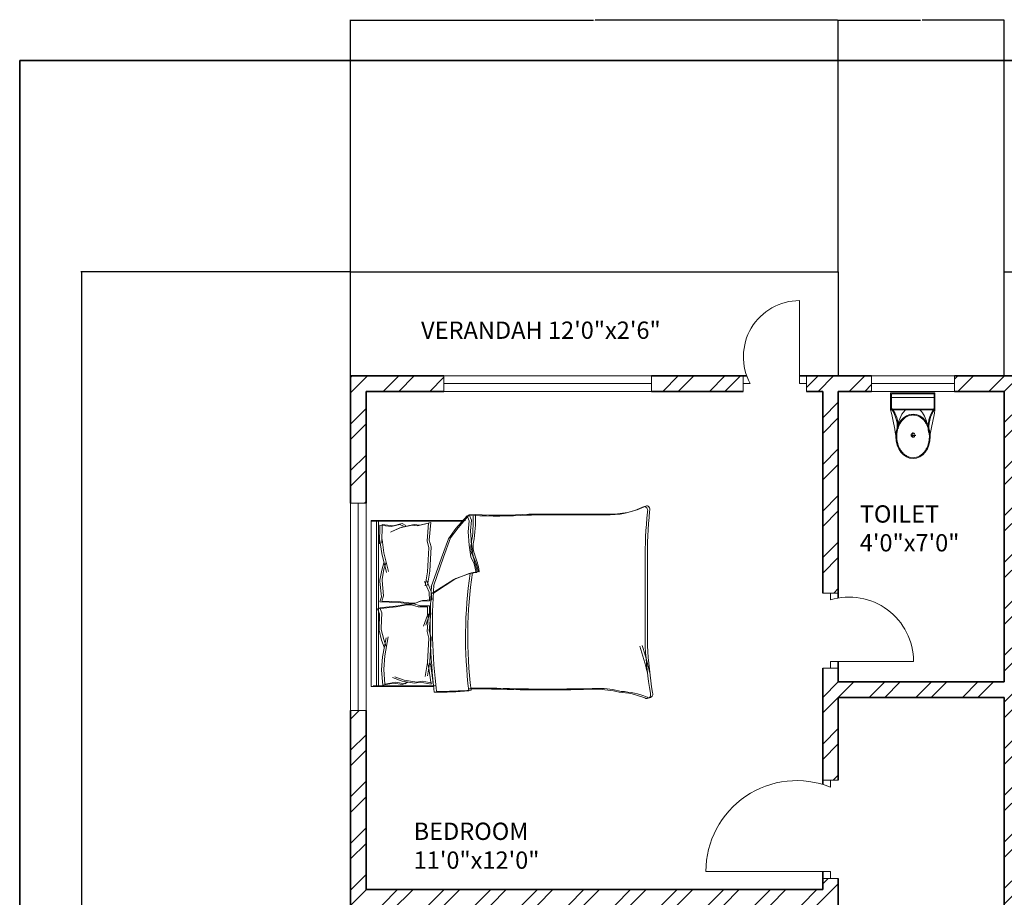
# Model space of a CAD drawing. Units: inches. Extents: x 1885 to 2748, y 783 to 2421.
# Tile 88 of 117: x 1885 to 2170, y 2167 to 2421. Entities that reach past the tile are written whole.
import ezdxf

# ---------------------------------------------------------------- set-up
doc = ezdxf.new("R2010")
doc.units = ezdxf.units.IN
for name, color, linetype, lineweight in [('A-ANNO-DIMS', 2, 'Continuous', 18), ('A-ANNO-TTLB', 7, 'Continuous', 35), ('A-AREA-IDEN', 7, 'Continuous', 18), ('A-DOOR', 31, 'Continuous', 18), ('A-FLOR-BALC', 7, 'Continuous', 25), ('A-FLOR-FIXT', 8, 'Continuous', 18), ('A-FURN', 8, 'Continuous', 13), ('A-GLAZ', 181, 'Continuous', 18), ('A-WALL', 7, 'Continuous', 35)]:
    doc.layers.add(name, color=color, linetype=linetype, lineweight=lineweight)
doc.layers.add('A-WALL-PATT', color=85, linetype='Continuous', lineweight=13, true_color=0x58ba48)
doc.styles.get("Standard").update_dxf_attribs({"font": 'arial.ttf'})
doc.dimstyles.get("Standard").update_dxf_attribs({"dimtxt": 0.18, "dimasz": 0.18, "dimexe": 0.18, "dimexo": 0.0625, "dimgap": 0.09, "dimtad": 0, "dimtih": 1, "dimtoh": 1, "dimdec": 4, "dimzin": 0, "dimdsep": 46, "dimtxsty": 'Standard', "dimcen": 0.09, "dimadec": 0, "dimazin": 0, "dimtfac": 1, "dimtdec": 4, "dimtofl": 0, "dimtmove": 0, "dimatfit": 3, "dimfxl": 1, "dimtolj": 1, "dimtzin": 0, "dimarcsym": 0})

# ---------------------------------------------------------------- blocks, each defined once
blk = doc.blocks.new('A$C31115884')
for p, q in [((283, 498), (223, 498)), ((258, 466), (258, 523)), ((0, 200), (0, 0)), ((520, 200), (0, 200)), ((10, 190), (10, 10)), ((510, 190), (10, 190)), ((510, 10), (510, 190)), ((520, 0), (520, 200)), ((510, 54), (0, 54)), ((10, 10), (510, 10)), ((0, 0), (520, 0))]:
    blk.add_line(p, q)
blk.add_circle((256, 496), 23.6)
for centre, radius, start, end in [((2778, -205), 2807, 165.4549, 171.7133), ((-295, 403), 365, 324.2091, 9.3499), ((-295, 403), 375, 324.2091, 9.3499), ((806, 403), 365, 170.6501, 215.7909), ((3237, 905), 2807, 188.2867, 194.5451), ((384, 406), 293, 190.2774, 224.1564), ((139, 406), 293, 315.8436, 2.6563), ((806, 403), 375, 179.2036, 215.7909)]:
    blk.add_arc(centre, radius, start, end)
blk.add_ellipse((256, 510), major_axis=(0, -261), ratio=0.772727)
blk.add_open_spline([(256, 259), (263, 259), (270, 260), (288, 262), (299, 265), (320, 273), (330, 278), (350, 291), (360, 299), (378, 316), (386, 326), (402, 347), (409, 358), (421, 383), (427, 395), (436, 422), (440, 436), (445, 465), (447, 480), (448, 509), (448, 524), (445, 553), (443, 568), (436, 596), (432, 610), (422, 636), (416, 649), (402, 672), (395, 683), (379, 703), (370, 712), (351, 728), (341, 735), (321, 746), (310, 751), (289, 757), (278, 759), (256, 761), (245, 761), (223, 757), (212, 754), (191, 746), (181, 741), (161, 728), (151, 720), (133, 703), (125, 693), (110, 672), (103, 660), (90, 636), (85, 623), (76, 596), (72, 582), (67, 553), (66, 538), (64, 509), (65, 494), (68, 465), (70, 450), (77, 422), (81, 408), (91, 382), (97, 370), (111, 346), (118, 335), (135, 316), (144, 307), (162, 291), (172, 284), (193, 273), (203, 269), (225, 262), (236, 260), (250, 259), (253, 259), (256, 259)], degree=3, knots=[0, 0, 0, 0, 0.110105, 0.110105, 0.285049, 0.285049, 0.459994, 0.459994, 0.634938, 0.634938, 0.809882, 0.809882, 0.984827, 0.984827, 1.159771, 1.159771, 1.334715, 1.334715, 1.50966, 1.50966, 1.684604, 1.684604, 1.859549, 1.859549, 2.034493, 2.034493, 2.209437, 2.209437, 2.384382, 2.384382, 2.559326, 2.559326, 2.73427, 2.73427, 2.909215, 2.909215, 3.084159, 3.084159, 3.259103, 3.259103, 3.434048, 3.434048, 3.608992, 3.608992, 3.783936, 3.783936, 3.958881, 3.958881, 4.133825, 4.133825, 4.30877, 4.30877, 4.483714, 4.483714, 4.658658, 4.658658, 4.833603, 4.833603, 5.008547, 5.008547, 5.183491, 5.183491, 5.358436, 5.358436, 5.53338, 5.53338, 5.708324, 5.708324, 5.883269, 5.883269, 6.058213, 6.058213, 6.233158, 6.233158, 6.283185, 6.283185, 6.283185, 6.283185])
blk = doc.blocks.new('BED-DOUBLE')
for p, q in [((0, 51.49), (0.64, 51.49)), ((0, 3.47), (0, 51.49)), ((0, 51.26), (26.61, 51.26)), ((0, 51.26), (26.61, 51.26)), ((0.64, 51.49), (27.25, 51.49)), ((0.64, 51.49), (27.25, 51.49)), ((1.54, 3.47), (1.54, 51.26)), ((1.54, 3.47), (1.54, 51.26)), ((2.18, 3.7), (2.18, 51.49)), ((2.18, 3.7), (2.18, 51.49)), ((27.75, 52.87), (24.5, 49.16)), ((27.75, 52.87), (24.5, 49.16)), ((28.39, 53.09), (25.14, 49.39)), ((28.39, 53.09), (25.14, 49.39)), ((29.49, 52.95), (27.75, 52.87, 3.87)), ((29.49, 52.95), (27.75, 52.87, 3.87)), ((28.37, 51.33), (27.75, 52.87)), ((28.37, 51.33), (27.75, 52.87)), ((28.06, 48.23), (28.37, 51.33)), ((28.06, 48.23), (28.37, 51.33)), ((30.13, 53.17), (28.39, 53.09, 3.87)), ((30.13, 53.17), (28.39, 53.09, 3.87)), ((29.01, 51.56), (28.39, 53.09)), ((29.01, 51.56), (28.39, 53.09)), ((28.7, 48.46), (29.01, 51.56)), ((28.7, 48.46), (29.01, 51.56)), ((2.56, 50.11), (2.46, 44.71)), ((2.56, 50.11), (2.46, 44.71)), ((2.56, 50.11), (5.77, 49.73)), ((2.56, 50.11), (5.77, 49.73)), ((3.2, 50.34), (3.1, 44.94)), ((3.2, 50.34), (3.1, 44.94)), ((3.2, 50.34), (6.41, 49.96)), ((3.2, 50.34), (6.41, 49.96)), ((8.26, 49.31), (5.58, 48.13)), ((8.26, 49.31), (5.58, 48.13)), ((5.77, 49.73), (8.34, 50.33)), ((5.77, 49.73), (8.34, 50.33)), ((8.9, 49.54), (6.22, 48.36)), ((8.9, 49.54), (6.22, 48.36)), ((6.41, 49.96), (8.98, 50.56)), ((6.41, 49.96), (8.98, 50.56)), ((11.83, 50.11), (8.26, 49.31)), ((11.83, 50.11), (8.26, 49.31)), ((8.34, 50.33), (9.39, 49.81)), ((8.34, 50.33), (9.39, 49.81)), ((12.47, 50.34), (8.9, 49.54)), ((12.47, 50.34), (8.9, 49.54)), ((8.98, 50.56), (10.03, 50.04)), ((8.98, 50.56), (10.03, 50.04)), ((13.44, 49.92), (11.83, 50.11)), ((13.44, 49.92), (11.83, 50.11)), ((14.08, 50.15), (12.47, 50.34)), ((14.08, 50.15), (12.47, 50.34)), ((16.58, 50.7), (13.44, 49.92)), ((16.58, 50.7), (13.44, 49.92)), ((17.22, 50.93), (14.08, 50.15)), ((17.22, 50.93), (14.08, 50.15)), ((16.17, 45.57), (16.58, 50.7)), ((16.17, 45.56), (16.58, 50.7)), ((16.81, 45.79), (17.22, 50.93)), ((16.81, 45.79), (17.22, 50.93)), ((24.5, 49.16), (22.33, 46.22)), ((24.5, 49.16), (22.33, 46.22)), ((25.14, 49.39), (22.97, 46.45)), ((25.14, 49.39), (22.97, 46.45)), ((29.01, 44.59), (28.7, 48.46)), ((29.01, 44.59), (28.7, 48.46)), ((2.46, 44.71), (2.55, 45.71)), ((2.46, 44.71), (2.55, 45.71)), ((2.55, 45.71), (3.07, 41.91)), ((2.55, 45.71), (3.07, 41.91)), ((3.1, 44.94), (3.19, 45.94)), ((3.1, 44.94), (3.19, 45.94)), ((3.19, 45.94), (3.71, 42.14)), ((3.19, 45.94), (3.71, 42.14)), ((16.73, 43.6), (16.17, 45.57)), ((16.73, 43.6), (16.17, 45.56)), ((17.37, 43.83), (16.81, 45.79)), ((17.37, 43.83), (16.81, 45.79)), ((22.33, 46.22), (20.32, 40.64)), ((22.33, 46.22), (20.32, 40.64)), ((22.97, 46.45), (20.96, 40.87)), ((22.97, 46.45), (20.96, 40.87)), ((28.37, 44.36), (28.06, 48.23)), ((28.37, 44.36), (28.06, 48.23)), ((16.3, 36.59), (16.73, 43.6)), ((16.3, 36.59), (16.73, 43.6)), ((16.94, 36.82), (17.37, 43.83)), ((16.94, 36.82), (17.37, 43.83)), ((28.83, 40.95), (28.37, 44.36)), ((28.83, 40.95), (28.37, 44.36)), ((29.47, 41.18), (29.01, 44.59)), ((29.47, 41.18), (29.01, 44.59)), ((3.07, 41.91), (4.43, 36.49)), ((3.07, 41.91), (4.43, 36.49)), ((3.71, 42.14), (5.07, 36.72)), ((3.71, 42.14), (5.07, 36.72)), ((20.32, 40.64), (17.39, 32.3)), ((20.32, 40.64), (17.39, 32.3)), ((20.96, 40.87), (18.03, 32.53)), ((20.96, 40.87), (18.03, 32.53)), ((29.76, 38.94), (28.83, 40.95)), ((29.76, 38.94), (28.83, 40.95)), ((30.4, 39.17), (29.47, 41.18)), ((30.4, 39.17), (29.47, 41.18)), ((79.89, 15.29), (79.89, 39.9)), ((79.89, 15.29), (79.89, 39.9)), ((3.08, 37.13), (2.54, 34.2)), ((3.08, 37.13), (2.54, 34.2)), ((3.68, 39.2), (3.08, 37.13)), ((3.68, 39.2), (3.08, 37.13)), ((3.72, 37.36), (3.18, 34.43)), ((3.72, 37.36), (3.18, 34.43)), ((4.32, 39.43), (3.72, 37.36)), ((4.32, 39.43), (3.72, 37.36)), ((30.38, 36.46), (29.76, 38.94)), ((30.38, 36.46), (29.76, 38.94)), ((31.02, 36.69), (30.4, 39.17)), ((31.02, 36.69), (30.4, 39.17)), ((79.25, 15.06), (79.25, 39.68)), ((79.25, 15.06), (79.25, 39.68)), ((2.54, 34.2), (2.56, 33.88)), ((2.54, 34.2), (2.56, 33.88)), ((3.18, 34.43), (3.2, 34.11)), ((3.18, 34.43), (3.2, 34.11)), ((15.63, 32.56), (16.3, 36.59)), ((15.63, 32.56), (16.3, 36.59)), ((16.27, 32.79), (16.94, 36.82)), ((16.27, 32.79), (16.94, 36.82)), ((17.39, 30.26), (23.88, 34.45)), ((17.39, 30.26), (23.88, 34.45)), ((18.03, 30.49), (24.52, 34.68)), ((18.03, 30.49), (24.52, 34.68)), ((23.88, 34.45), (28.37, 36.15)), ((23.88, 34.45), (28.37, 36.15)), ((24.52, 34.68), (29.01, 36.38)), ((24.52, 34.68), (29.01, 36.38)), ((28.37, 36.15), (30.38, 36.46)), ((28.37, 36.15), (30.38, 36.46)), ((29.01, 36.38), (31.02, 36.69)), ((29.01, 36.38), (31.02, 36.69)), ((2.56, 33.88), (2.98, 29.45)), ((2.56, 33.88), (2.98, 29.45)), ((3.2, 34.11), (3.62, 29.68)), ((3.2, 34.11), (3.62, 29.68)), ((16.74, 30.75), (15.46, 33.82)), ((16.74, 30.75), (15.46, 33.82)), ((17.38, 30.98), (16.1, 34.05)), ((17.38, 30.98), (16.1, 34.05)), ((2.98, 29.45), (2.5, 27.98)), ((2.98, 29.45), (2.5, 27.98)), ((3.62, 29.68), (3.13, 28.2)), ((3.62, 29.68), (3.13, 28.2)), ((14.86, 28.36), (17.54, 28.52)), ((14.86, 28.36), (17.54, 28.52)), ((16.9, 28.3), (16.74, 30.75)), ((16.9, 28.3), (16.74, 30.75)), ((17.54, 28.52), (17.38, 30.98)), ((17.54, 28.52), (17.38, 30.98)), ((1.87, 25.98), (7.22, 26.56)), ((1.87, 25.98), (7.22, 26.56)), ((2.45, 24.54), (1.87, 25.98)), ((2.45, 24.54), (1.87, 25.98)), ((2.5, 27.98), (7.87, 27.73)), ((2.5, 27.98), (7.87, 27.73)), ((2.51, 26.21), (7.86, 26.79)), ((2.51, 26.21), (7.86, 26.79)), ((3.09, 24.76), (2.51, 26.21)), ((3.09, 24.76), (2.51, 26.21)), ((3.13, 28.2), (8.51, 27.96)), ((3.13, 28.2), (8.51, 27.96)), ((7.22, 26.56), (10.4, 27.14)), ((7.22, 26.56), (10.4, 27.14)), ((7.86, 26.79), (11.04, 27.37)), ((7.86, 26.79), (11.04, 27.37)), ((7.87, 27.73), (11.08, 27.35)), ((7.87, 27.73), (11.08, 27.35)), ((8.51, 27.96), (11.72, 27.58)), ((8.51, 27.96), (11.72, 27.58)), ((10.4, 27.14), (11.71, 27.14)), ((10.4, 27.14), (11.71, 27.14)), ((11.04, 27.37), (12.35, 27.37)), ((11.04, 27.37), (12.35, 27.37)), ((11.08, 27.35), (12.38, 27.43)), ((11.08, 27.35), (12.38, 27.43)), ((11.71, 27.14), (13.59, 26.56)), ((11.71, 27.14), (13.59, 26.56)), ((11.72, 27.58), (13.02, 27.66)), ((11.72, 27.58), (13.02, 27.66)), ((12.35, 27.37), (14.22, 26.79)), ((12.35, 27.37), (14.22, 26.79)), ((12.38, 27.43), (14.22, 28.13)), ((12.38, 27.43), (14.22, 28.13)), ((13.02, 27.66), (14.86, 28.36)), ((13.02, 27.66), (14.86, 28.36)), ((13.59, 26.56), (16.27, 26.56)), ((13.59, 26.56), (16.27, 26.56)), ((14.22, 28.13), (16.9, 28.3)), ((14.22, 28.13), (16.9, 28.3)), ((14.22, 26.79), (16.91, 26.79)), ((14.22, 26.79), (16.91, 26.79)), ((16.27, 26.56), (16.27, 24.1)), ((16.27, 26.56), (16.27, 24.1)), ((16.91, 26.79), (16.91, 24.33)), ((16.91, 26.79), (16.91, 24.33)), ((2.31, 20.09), (2.45, 24.54)), ((2.31, 20.09), (2.45, 24.54)), ((2.95, 20.32), (3.09, 24.76)), ((2.95, 20.32), (3.09, 24.76)), ((16.27, 24.1), (15.18, 20.96)), ((16.27, 24.1), (15.18, 20.96)), ((16.91, 24.33), (15.82, 21.19)), ((16.91, 24.33), (15.82, 21.19)), ((16.17, 19.38), (16.58, 24.51)), ((16.17, 19.38), (16.58, 24.51)), ((16.81, 19.61), (17.22, 24.74)), ((16.81, 19.61), (17.22, 24.74)), ((2.31, 19.77), (2.31, 20.09)), ((2.31, 19.77), (2.31, 20.09)), ((2.95, 20), (2.95, 20.32)), ((2.95, 20), (2.95, 20.32)), ((3.67, 17.11), (2.95, 20)), ((3.67, 17.11), (2.95, 20)), ((3.03, 16.88), (2.31, 19.77)), ((3.03, 16.88), (2.31, 19.77)), ((3.32, 12.11), (4.33, 17.6)), ((3.32, 12.11), (4.33, 17.6)), ((4.39, 15.08), (3.67, 17.11)), ((4.39, 15.08), (3.67, 17.11)), ((3.96, 12.34), (4.97, 17.83)), ((3.96, 12.34), (4.97, 17.83)), ((16.73, 17.42), (16.17, 19.38)), ((16.73, 17.42), (16.17, 19.38)), ((16.3, 10.41), (16.73, 17.42)), ((16.3, 10.41), (16.73, 17.42)), ((17.37, 17.65), (16.81, 19.61)), ((17.37, 17.65), (16.81, 19.61)), ((16.94, 10.64), (17.37, 17.65)), ((16.94, 10.64), (17.37, 17.65)), ((3.75, 14.85), (3.03, 16.88)), ((3.75, 14.85), (3.03, 16.88)), ((3.03, 8.28), (3.32, 12.11)), ((3.03, 8.28), (3.32, 12.11)), ((3.67, 8.51), (3.96, 12.34)), ((3.67, 8.51), (3.96, 12.34)), ((15.63, 6.38), (16.3, 10.41)), ((15.63, 6.38), (16.3, 10.41)), ((16.27, 6.61), (16.94, 10.64)), ((16.27, 6.61), (16.94, 10.64)), ((16.3, 10.41), (16.62, 9.28)), ((16.3, 10.41), (16.62, 9.28)), ((16.62, 9.28), (17.34, 4.18)), ((16.62, 9.28), (17.34, 4.18)), ((16.94, 10.64), (17.26, 9.51)), ((16.94, 10.64), (17.26, 9.51)), ((17.26, 9.51), (17.98, 4.41)), ((17.26, 9.51), (17.98, 4.41)), ((3.01, 8.18), (3.03, 8.28)), ((3.01, 8.18), (3.03, 8.28)), ((3.34, 3.9), (3.01, 8.18)), ((3.34, 3.9), (3.01, 8.18)), ((3.65, 8.41), (3.67, 8.51)), ((3.65, 8.41), (3.67, 8.51)), ((3.98, 4.13), (3.65, 8.41)), ((3.98, 4.13), (3.65, 8.41)), ((8.96, 5.05), (6.21, 6.06)), ((8.96, 5.05), (6.21, 6.06)), ((9.6, 5.28), (6.85, 6.29)), ((9.6, 5.28), (6.85, 6.29)), ((18.11, 3.47), (0, 3.47)), ((18.11, 3.47), (0, 3.47)), ((18.75, 3.7), (0.64, 3.7)), ((18.75, 3.7), (0.64, 3.7)), ((3.32, 3.89), (6.5, 4.47)), ((3.32, 3.89), (6.5, 4.47)), ((3.96, 4.12), (7.14, 4.7)), ((3.96, 4.12), (7.14, 4.7)), ((6.5, 4.47), (9.1, 4.04)), ((6.5, 4.47), (9.1, 4.04)), ((7.14, 4.7), (9.74, 4.27)), ((7.14, 4.7), (9.74, 4.27)), ((12.57, 4.47), (8.96, 5.05)), ((12.57, 4.47), (8.96, 5.05)), ((9.1, 4.04), (10.12, 4.62)), ((9.1, 4.04), (10.12, 4.62)), ((13.21, 4.7), (9.6, 5.28)), ((13.21, 4.7), (9.6, 5.28)), ((9.74, 4.27), (10.75, 4.84)), ((9.74, 4.27), (10.75, 4.84)), ((14.16, 4.76), (12.57, 4.47)), ((14.16, 4.76), (12.57, 4.47)), ((14.8, 4.99), (13.21, 4.7)), ((14.8, 4.99), (13.21, 4.7)), ((17.34, 4.18), (14.16, 4.76)), ((17.34, 4.18), (14.16, 4.76)), ((17.98, 4.41), (14.8, 4.99)), ((17.98, 4.41), (14.8, 4.99))]:
    blk.add_line(p, q)
for centre, radius, start, end in [((68.67, 76.16), 23.07, 267.4714, 296.4681), ((68.67, 76.16), 23.07, 267.4714, 296.4681), ((69.31, 76.38), 23.07, 267.4714, 296.4681), ((69.31, 76.38), 23.07, 267.4714, 296.4681), ((78.87, 54.41), 1.1, 332.6588, 86.02), ((78.87, 54.41), 1.1, 332.6588, 86.02), ((79.51, 54.64), 1.1, 332.6588, 86.02), ((79.51, 54.64), 1.1, 332.6588, 86.02), ((212.92, 41.38), 133.04, 174.4998, 180.6351), ((212.92, 41.38), 133.04, 174.4998, 180.6351), ((-6.65, 51.33), 36.18, 349.8763, 2.5657), ((-6.65, 51.33), 36.18, 349.8763, 2.5657), ((36.32, 182.26), 129.5, 266.9791, 273.8365), ((36.32, 182.26), 129.5, 266.9791, 273.8365), ((-6.01, 51.55), 36.18, 349.8763, 2.5657), ((-6.01, 51.55), 36.18, 349.8763, 2.5657), ((36.96, 182.49), 129.5, 266.9791, 273.8365), ((36.96, 182.49), 129.5, 266.9791, 273.8365), ((67.83, -4508.74), 4561.86, 90.00217, 90.28689), ((67.83, -4508.75), 4561.86, 90.00217, 90.28689), ((68.46, -4508.52), 4561.86, 90.00217, 90.28689), ((68.46, -4508.52), 4561.86, 90.00217, 90.28689), ((212.28, 41.15), 133.04, 174.4998, 180.6351), ((212.28, 41.15), 133.04, 174.4998, 180.6351), ((35.07, 43.74), 6.22, 168.6608, 203.7384), ((35.07, 43.74), 6.22, 168.6608, 203.7384), ((35.71, 43.97), 6.22, 168.6608, 203.7384), ((35.71, 43.97), 6.22, 168.6608, 203.7384), ((1.49, 31.15), 29.65, 10.6617, 19.8806), ((1.49, 31.15), 29.65, 10.6617, 19.8806), ((2.13, 31.38), 29.65, 10.6617, 19.8806), ((2.13, 31.38), 29.65, 10.6617, 19.8806), ((156.32, 17.75), 129.02, 171.7845, 186.9006), ((156.32, 17.75), 129.02, 171.7845, 186.9006), ((156.96, 17.98), 129.02, 171.7845, 186.9006), ((156.96, 17.98), 129.02, 171.7845, 186.9006), ((30.44, 36.64), 0.185, 250.2464, 1.1377), ((30.44, 36.63), 0.185, 250.2464, 1.1377), ((31.08, 36.86), 0.185, 250.2464, 1.1377), ((31.08, 36.86), 0.185, 250.2464, 1.1377), ((182.06, 21.36), 164.97, 176.0865, 186.7821), ((182.06, 21.36), 164.97, 176.0865, 186.7821), ((182.7, 21.59), 164.97, 176.0865, 186.7821), ((182.7, 21.59), 164.97, 176.0865, 186.7821), ((-23.71, -17.22), 106.46, 13.3832, 17.7053), ((-23.71, -17.22), 106.46, 13.3832, 17.7053), ((-23.07, -16.99), 106.46, 13.3832, 17.7053), ((-23.07, -16.99), 106.46, 13.3832, 17.7053), ((200.84, 21.43), 121.76, 182.9958, 189.4091), ((200.84, 21.43), 121.76, 182.9958, 189.4091), ((201.48, 21.65), 121.76, 182.9958, 189.4091), ((201.48, 21.65), 121.76, 182.9958, 189.4091), ((31.82, -167.08), 170.11, 88.4762, 91.0082), ((31.82, -167.08), 170.11, 88.4762, 91.0082), ((51.26, 485.05), 482.31, 268.2277, 271.7185), ((51.26, 485.05), 482.31, 268.2277, 271.7185), ((65.16, -26.67), 29.63, 76.0648, 88.9113), ((65.16, -26.67), 29.63, 76.0648, 88.9113), ((20.1, 85.16), 83.31, 268.7218, 275.604), ((20.1, 85.16), 83.31, 268.7218, 275.604), ((20.74, 85.39), 83.31, 268.7218, 275.604), ((20.74, 85.39), 83.31, 268.7218, 275.604), ((31.18, -167.31), 170.11, 88.4762, 91.0082), ((31.18, -167.31), 170.11, 88.4762, 91.0082), ((50.62, 484.82), 482.31, 268.2277, 271.7185), ((50.62, 484.82), 482.31, 268.2277, 271.7185), ((64.52, -26.9), 29.63, 76.0648, 88.9113), ((64.52, -26.9), 29.63, 76.0648, 88.9113), ((70.28, -21.66), 23.56, 67.9751, 86.652), ((70.28, -21.66), 23.56, 67.9751, 86.652), ((70.92, -21.43), 23.56, 67.9751, 86.652), ((70.92, -21.43), 23.56, 67.9751, 86.652), ((79.72, 1.09), 1.09, 236.1736, 23.4781), ((79.72, 1.09), 1.09, 236.1736, 23.4781), ((80.36, 1.31), 1.09, 236.1736, 23.4781), ((80.36, 1.31), 1.09, 236.1736, 23.4781)]:
    blk.add_arc(centre, radius, start, end)
blk = doc.blocks.new('WIN-60')
for p, q in [((0, 60), (4.5, 60)), ((0, 60), (0, 0)), ((4.5, 60), (2.25, 60)), ((2.25, 60), (2.25, 0)), ((4.5, 0), (4.5, 60)), ((2.25, 0), (0, 0)), ((0, 0), (4.5, 0))]:
    blk.add_line(p, q)
blk = doc.blocks.new('WIN-60-ALT')
for p, q in [((0, 60), (4.5, 60)), ((0, 60), (0, 0)), ((4.5, 60), (2.25, 60)), ((2.25, 60), (2.25, 0)), ((4.5, 0), (4.5, 60)), ((4.5, 0), (0, 0)), ((2.25, 0), (4.5, 0))]:
    blk.add_line(p, q)
blk = doc.blocks.new('*D48')
at = {"layer": 'A-ANNO-DIMS', "color": 0, "lineweight": -2, "transparency": 16777216}
for p, q in [((1980.71, 2348.01), (1902.84, 2348.01)), ((1903.02, 2347.83), (1903.02, 2114.94)), ((1903.02, 1881.69), (1903.02, 2114.57)), ((2016.71, 1881.51), (1902.84, 1881.51))]:
    blk.add_line(p, q, dxfattribs=at)
at = {"layer": 'A-ANNO-DIMS', "color": 0, "transparency": 16777216}
for points in [[(1902.99, 2347.83), (1903.05, 2347.83), (1903.02, 2348.01)], [(1902.99, 1881.69), (1903.05, 1881.69), (1903.02, 1881.51)]]:
    blk.add_solid(points, dxfattribs=at)
at = {"layer": 'Defpoints', "color": 0, "transparency": 16777216}
for p in [(1903.02, 2348.01), (1980.77, 2348.01), (2016.77, 1881.51)]:
    blk.add_point(p, dxfattribs=at)
at = {"layer": 'A-ANNO-DIMS', "color": 0, "transparency": 16777216, "insert": (1903.02, 2114.76), "char_height": 0.18, "attachment_point": 5}
blk.add_mtext('\\A1;466.5', dxfattribs=at)
blk = doc.blocks.new('*D49')
at = {"layer": 'A-ANNO-DIMS', "color": 0, "lineweight": -2, "transparency": 16777216}
for p, q in [((1980.77, 2348.07), (1980.77, 2420.94)), ((1980.95, 2420.76), (2051.01, 2420.76)), ((2121.59, 2420.76), (2051.54, 2420.76)), ((2121.77, 2348.07), (2121.77, 2420.94))]:
    blk.add_line(p, q, dxfattribs=at)
at = {"layer": 'A-ANNO-DIMS', "color": 0, "transparency": 16777216}
for points in [[(1980.95, 2420.79), (1980.95, 2420.73), (1980.77, 2420.76)], [(2121.59, 2420.79), (2121.59, 2420.73), (2121.77, 2420.76)]]:
    blk.add_solid(points, dxfattribs=at)
at = {"layer": 'Defpoints', "color": 0, "transparency": 16777216}
for p in [(2121.77, 2420.76), (1980.77, 2348.01), (2121.77, 2348.01)]:
    blk.add_point(p, dxfattribs=at)
at = {"layer": 'A-ANNO-DIMS', "color": 0, "transparency": 16777216, "insert": (2051.27, 2420.76), "char_height": 0.18, "attachment_point": 5}
blk.add_mtext('\\A1;141', dxfattribs=at)
blk = doc.blocks.new('*D50')
at = {"layer": 'A-ANNO-DIMS', "color": 0, "lineweight": -2, "transparency": 16777216}
for p, q in [((2121.77, 2348.07), (2121.77, 2420.94)), ((2121.95, 2420.76), (2145.55, 2420.76)), ((2169.59, 2420.76), (2146, 2420.76)), ((2169.77, 2348.07), (2169.77, 2420.94))]:
    blk.add_line(p, q, dxfattribs=at)
at = {"layer": 'A-ANNO-DIMS', "color": 0, "transparency": 16777216}
for points in [[(2121.95, 2420.79), (2121.95, 2420.73), (2121.77, 2420.76)], [(2169.59, 2420.79), (2169.59, 2420.73), (2169.77, 2420.76)]]:
    blk.add_solid(points, dxfattribs=at)
at = {"layer": 'Defpoints', "color": 0, "transparency": 16777216}
for p in [(2169.77, 2420.76), (2121.77, 2348.01), (2169.77, 2348.01)]:
    blk.add_point(p, dxfattribs=at)
at = {"layer": 'A-ANNO-DIMS', "color": 0, "transparency": 16777216, "insert": (2145.77, 2420.76), "char_height": 0.18, "attachment_point": 5}
blk.add_mtext('\\A1;48', dxfattribs=at)

msp = doc.modelspace()

# ---------------------------------------------------------------- hatches: boundary and pattern name
at = {"layer": 'A-WALL-PATT'}
h = msp.add_hatch(dxfattribs=at)
h.set_pattern_fill('ANSI32', color=256)
h.paths.add_polyline_path([(2007.77, 2318.01), (1980.77, 2318.01), (1980.77, 2281.22), (1985.27, 2281.22), (1985.27, 2313.51), (2007.77, 2313.51), (2007.77, 2315.76)])
h.paths.add_polyline_path([(2094.32, 2318.01), (2067.77, 2318.01), (2067.77, 2313.51), (2094.32, 2313.51), (2094.32, 2315.76)])
h.paths.add_polyline_path([(2131.37, 2315.76), (2131.37, 2318.01), (2131.19, 2318.01), (2112.61, 2318.01), (2112.61, 2313.51), (2117.27, 2313.51), (2117.27, 2255.2), (2121.77, 2255.2), (2121.77, 2313.51), (2131.37, 2313.51)])
h.paths.add_polyline_path([(2190.51, 2318.01), (2155.37, 2318.01), (2155.37, 2313.51), (2169.77, 2313.51), (2169.77, 2229.51), (2121.77, 2229.51), (2121.77, 2233.45), (2119.52, 2233.45), (2117.27, 2233.45), (2117.27, 2201.1), (2121.77, 2201.1), (2121.77, 2225.01), (2169.77, 2225.01), (2169.77, 2165.01), (2306.27, 2165.01), (2306.27, 2066.01), (2310.77, 2066.01), (2344.27, 2066.01), (2486.27, 2066.01), (2486.27, 1886.01), (2483.02, 1886.01), (2483.02, 1881.51), (2486.27, 1881.51), (2486.27, 1880.68), (2490.77, 1880.68), (2490.77, 2070.51), (2344.27, 2070.51), (2310.77, 2070.51), (2310.77, 2165.01), (2310.77, 2173.64), (2308.52, 2173.64), (2306.27, 2173.64), (2306.27, 2169.51), (2174.27, 2169.51), (2174.27, 2313.51), (2190.51, 2313.51), (2190.51, 2315.76)])
h.paths.add_polyline_path([(1985.27, 2221.22), (1980.77, 2221.22), (1980.77, 2165.01), (1992.77, 2165.01), (1992.77, 2141.93), (1997.27, 2141.93), (1997.27, 2165.01), (2117.27, 2165.01), (2117.27, 2163.13), (2121.77, 2163.13), (2121.77, 2172.73), (2119.52, 2172.73), (2117.27, 2172.73), (2117.27, 2169.51), (1985.27, 2169.51)])
h.paths.add_polyline_path([(1997.27, 2105.93), (1992.77, 2105.93), (1992.77, 2070.51), (2016.77, 2070.51), (2016.77, 2059.12), (2019.02, 2059.12), (2021.27, 2059.12), (2021.27, 2070.51), (2117.27, 2070.51), (2117.27, 2022.51), (2114.42, 2022.51), (2114.42, 2018.01), (2123.63, 2018.01), (2123.63, 2020.26), (2123.63, 2022.51), (2121.77, 2022.51), (2121.77, 2142.59), (2119.52, 2142.59), (2117.27, 2142.59), (2117.27, 2075.01), (1997.27, 2075.01)])
h.paths.add_polyline_path([(2092.03, 2020.26), (2092.03, 2022.51), (2021.27, 2022.51), (2021.27, 2035.12), (2016.77, 2035.12), (2016.77, 2018.01), (2016.77, 1978.78), (2021.27, 1978.78), (2021.27, 2018.01), (2092.03, 2018.01)])
h.paths.add_polyline_path([(2260.94, 2022.51), (2153.1, 2022.51), (2153.1, 2020.26), (2153.1, 2018.01), (2155.27, 2018.01), (2155.27, 1886.01), (2107.63, 1886.01), (2107.63, 1881.51), (2182.91, 1881.51), (2182.91, 1883.76), (2182.91, 1886.01), (2159.77, 1886.01), (2159.77, 2018.01), (2260.94, 2018.01), (2260.94, 2020.26)])
h.paths.add_polyline_path([(2047.63, 1883.76), (2047.63, 1886.01), (2021.27, 1886.01), (2021.27, 1918.78), (2019.02, 1918.78), (2016.77, 1918.78), (2016.77, 1881.51), (2047.63, 1881.51)])
h.paths.add_polyline_path([(2306.36, 1883.76), (2306.36, 1886.01), (2296.27, 1886.01), (2296.27, 1982.01), (2316.54, 1982.01), (2316.54, 1984.26), (2316.54, 1986.51), (2296.27, 1986.51), (2296.27, 2022.51), (2289.28, 2022.51), (2289.28, 2018.01), (2291.77, 2018.01), (2291.77, 1886.01), (2242.91, 1886.01), (2242.91, 1881.51), (2306.36, 1881.51)], flags=17)
h.paths.add_polyline_path([(1985.27, 1843.01), (2021.6, 1843.01), (2021.53, 1845.44), (2021.48, 1847.51), (1980.77, 1847.51), (1980.77, 1809.45), (1985.27, 1809.45)])
h.paths.add_polyline_path([(2131.48, 1845.26), (2131.48, 1847.51), (2081.53, 1847.51), (2081.53, 1843.01), (2117.27, 1843.01), (2117.27, 1784.15), (2119.52, 1784.15), (2121.77, 1784.15), (2121.77, 1843.01), (2131.48, 1843.01)])
h.paths.add_polyline_path([(2203.89, 1847.51), (2155.48, 1847.51), (2155.48, 1843.01), (2169.77, 1843.01), (2169.77, 1759.01), (2121.77, 1759.01), (2121.77, 1761.46), (2117.27, 1761.46), (2117.27, 1730.43), (2121.77, 1730.43), (2121.77, 1754.51), (2177.42, 1754.51), (2177.42, 1756.76), (2177.42, 1759.01), (2174.27, 1759.01), (2174.27, 1843.01), (2203.89, 1843.01)])
h.paths.add_polyline_path([(2335.55, 1845.26), (2335.55, 1847.51), (2239.89, 1847.51), (2239.89, 1843.01), (2306.27, 1843.01), (2306.27, 1759.01), (2199.49, 1759.01), (2199.49, 1754.51), (2310.77, 1754.51), (2310.77, 1843.01), (2335.55, 1843.01)])
h.paths.add_polyline_path([(2348.77, 2022.51), (2344.27, 2022.51), (2344.27, 1986.51), (2341.68, 1986.51), (2341.68, 1982.01), (2344.27, 1982.01), (2344.27, 1886.01), (2330.36, 1886.01), (2330.36, 1881.51), (2361.63, 1881.51), (2361.63, 1883.76), (2361.63, 1886.01), (2348.77, 1886.01)], flags=17)
h.paths.add_polyline_path([(2283.25, 2315.76), (2283.25, 2318.01), (2238.51, 2318.01), (2238.51, 2313.51), (2283.25, 2313.51)], flags=17)
h.paths.add_polyline_path([(2363.27, 2348.01), (2388.68, 2348.01), (2388.68, 2350.26), (2388.68, 2352.51), (2358.77, 2352.51), (2358.77, 2348.01), (2358.77, 2318.01), (2344.48, 2318.01), (2344.48, 2313.51), (2358.77, 2313.51), (2358.77, 2229.51), (2310.77, 2229.51), (2310.77, 2231.95), (2306.27, 2231.95), (2306.27, 2205.61), (2310.77, 2205.61), (2310.77, 2225.01), (2358.77, 2225.01), (2358.77, 2211.51), (2452.33, 2211.51), (2452.33, 2213.76), (2452.33, 2216.01), (2363.27, 2216.01), (2363.27, 2318.01)])
h.paths.add_polyline_path([(2310.77, 2313.51), (2320.48, 2313.51), (2320.48, 2315.76), (2320.48, 2318.01), (2302.73, 2318.01), (2302.73, 2313.51), (2306.27, 2313.51), (2306.27, 2251.08), (2310.77, 2251.08)], flags=17)
h.paths.add_polyline_path([(2490.77, 2352.51), (2486.27, 2352.51), (2448.68, 2352.51), (2448.68, 2348.01), (2486.27, 2348.01), (2486.27, 2318.01), (2486.27, 2216.01), (2481.78, 2216.01), (2481.78, 2211.51), (2486.27, 2211.51), (2486.27, 2165.01), (2493.29, 2165.01), (2493.29, 2167.26), (2493.29, 2169.51), (2490.77, 2169.51), (2490.77, 2313.51), (2494.43, 2313.51), (2494.43, 2318.01), (2490.77, 2318.01)])
h.paths.add_polyline_path([(2534.65, 2318.01), (2515.69, 2318.01), (2515.69, 2313.51), (2534.65, 2313.51), (2534.65, 2315.76)])
h.paths.add_polyline_path([(2618.27, 2318.01), (2594.65, 2318.01), (2594.65, 2313.51), (2613.77, 2313.51), (2613.77, 2281.71), (2618.27, 2281.71)])
h.paths.add_polyline_path([(2618.27, 2221.71), (2613.77, 2221.71), (2613.77, 2169.51), (2554.02, 2169.51), (2554.02, 2165.01), (2613.77, 2165.01), (2613.77, 2152.88), (2618.27, 2152.88)])
h.paths.add_polyline_path([(2618.27, 2128.88), (2616.02, 2128.88), (2613.77, 2128.88), (2613.77, 2117.01), (2529.77, 2117.01), (2529.77, 2165.01), (2532.85, 2165.01), (2532.85, 2169.51), (2522.87, 2169.51), (2522.87, 2165.01), (2525.27, 2165.01), (2525.27, 2117.01), (2525.27, 2112.51), (2525.27, 2108.58), (2529.77, 2108.58), (2529.77, 2112.51), (2613.77, 2112.51), (2613.77, 2080.19), (2618.27, 2080.19)])
h.paths.add_polyline_path([(2618.27, 2044.19), (2616.02, 2044.19), (2613.77, 2044.19), (2613.77, 2015.51), (2529.77, 2015.51), (2529.77, 2088.58), (2527.52, 2088.58), (2525.27, 2088.58), (2525.27, 2011.01), (2613.77, 2011.01), (2613.77, 1956.75), (2618.27, 1956.75)])
h.paths.add_polyline_path([(2618.27, 1881.51), (2618.27, 1896.75), (2613.77, 1896.75), (2613.77, 1881.51), (2613.77, 1847.51), (2592.71, 1847.51), (2592.71, 1843.01), (2613.77, 1843.01), (2613.77, 1765.01), (2613.77, 1760.51), (2609.62, 1760.51), (2609.62, 1756.01), (2613.77, 1756.01), (2613.77, 1660.01), (2608.54, 1660.01), (2608.54, 1655.51), (2613.77, 1655.51), (2613.77, 1508.16), (2618.27, 1508.16)])
h.paths.add_polyline_path([(2565.77, 1843.01), (2569, 1843.01), (2569, 1847.51), (2490.77, 1847.51), (2490.77, 1849.7), (2488.52, 1849.7), (2486.27, 1849.7), (2486.27, 1847.51), (2477.27, 1847.51), (2477.27, 1838.51), (2477.27, 1821.49), (2486.27, 1821.49), (2486.27, 1838.51), (2561.27, 1838.51), (2561.27, 1765.01), (2486.27, 1765.01), (2486.27, 1786.16), (2477.27, 1786.16), (2477.27, 1765.01), (2477.27, 1756.01), (2486.27, 1756.01), (2565.77, 1756.01), (2585.62, 1756.01), (2585.62, 1758.26), (2585.62, 1760.51), (2565.77, 1760.51), (2565.77, 1765.01)])
h.paths.add_polyline_path([(2486.27, 1651.01), (2561.27, 1651.01), (2561.27, 1567.01), (2486.27, 1567.01), (2486.27, 1591.32), (2477.27, 1591.32), (2477.27, 1567.01), (2477.27, 1558.01), (2477.27, 1555.44), (2481.77, 1555.44), (2481.77, 1558.01), (2568.65, 1558.01), (2568.65, 1560.26), (2568.65, 1562.51), (2565.77, 1562.51), (2565.77, 1655.51), (2584.54, 1655.51), (2584.54, 1657.76), (2584.54, 1660.01), (2565.77, 1660.01), (2486.27, 1660.01), (2477.27, 1660.01), (2477.27, 1651.01), (2477.27, 1632.99), (2486.27, 1632.99)])
h.paths.add_polyline_path([(2449.97, 1883.76), (2449.97, 1886.01), (2421.63, 1886.01), (2421.63, 1881.51), (2449.97, 1881.51)], flags=17)
h.paths.add_polyline_path([(2447.27, 1847.51), (2395.55, 1847.51), (2395.55, 1843.01), (2442.77, 1843.01), (2442.77, 1809.27), (2447.27, 1809.27)])
h.paths.add_polyline_path([(1985.27, 1749.45), (1980.77, 1749.45), (1980.77, 1694.5), (1985.27, 1694.5), (1985.27, 1694.51), (1986.9, 1694.51), (1986.9, 1697.78), (1986.9, 1699.01), (1985.27, 1699.01)])
h.paths.add_polyline_path([(2152.77, 1699.01), (2121.77, 1699.01), (2121.77, 1703.67), (2119.52, 1703.67), (2117.27, 1703.67), (2117.27, 1699.01), (2009.22, 1699.01), (2009.22, 1694.51), (2148.27, 1694.51), (2148.27, 1692.63), (2152.77, 1692.63)])
h.paths.add_polyline_path([(2016.27, 1694.51), (2011.77, 1694.51), (2011.77, 1558.01), (2040.81, 1558.01), (2040.81, 1560.26), (2040.81, 1562.51), (2016.27, 1562.51)])
h.paths.add_polyline_path([(2152.77, 1663.02), (2150.52, 1663.02), (2148.27, 1663.02), (2148.27, 1562.51), (2100.81, 1562.51), (2100.81, 1558.01), (2165.12, 1558.01), (2165.12, 1560.26), (2165.12, 1562.51), (2152.77, 1562.51), (2152.77, 1610.51), (2224.77, 1610.51), (2224.77, 1607.99), (2229.27, 1607.99), (2229.27, 1615.01), (2152.77, 1615.01)])
h.paths.add_polyline_path([(2238.61, 1560.26), (2238.61, 1562.51), (2229.27, 1562.51), (2229.27, 1588.76), (2227.02, 1588.76), (2224.77, 1588.77), (2224.77, 1562.51), (2189.12, 1562.51), (2189.12, 1558.01), (2238.61, 1558.01)])
h.paths.add_polyline_path([(2336.02, 1560.26), (2336.02, 1562.51), (2310.77, 1562.51), (2310.77, 1656.35), (2308.52, 1656.35), (2306.27, 1656.35), (2306.27, 1562.51), (2286.61, 1562.51), (2286.61, 1558.01), (2336.02, 1558.01)])
h.paths.add_polyline_path([(2447.27, 1690.97), (2445.02, 1690.97), (2442.77, 1690.97), (2442.77, 1687.01), (2306.27, 1687.01), (2306.27, 1680.75), (2310.77, 1680.75), (2310.77, 1682.51), (2442.77, 1682.51), (2442.77, 1562.51), (2396.02, 1562.51), (2396.02, 1558.01), (2447.27, 1558.01)])
h.paths.add_polyline_path([(2447.27, 1749.27), (2445.02, 1749.27), (2442.77, 1749.27), (2442.77, 1717.23), (2447.27, 1717.23)])
h.paths.add_polyline_path([(2044.67, 1521.76), (2044.67, 1524.01), (2007.27, 1524.01), (2007.27, 1503.49), (2009.52, 1503.49), (2011.77, 1503.49), (2011.77, 1519.51), (2044.67, 1519.51)])
h.paths.add_polyline_path([(2177.97, 1521.76), (2177.97, 1524.01), (2104.67, 1524.01), (2104.67, 1519.51), (2145.77, 1519.51), (2145.77, 1387.51), (2143.37, 1387.51), (2143.37, 1383.01), (2251.59, 1383.01), (2251.59, 1385.26), (2251.59, 1387.51), (2150.27, 1387.51), (2150.27, 1519.51), (2177.97, 1519.51)])
h.paths.add_polyline_path([(2298.7, 1524.01), (2237.97, 1524.01), (2237.97, 1519.51), (2282.27, 1519.51), (2282.27, 1387.51), (2279.68, 1387.51), (2279.68, 1383.01), (2286.77, 1383.01), (2286.77, 1419.01), (2312.45, 1419.01), (2312.45, 1421.26), (2312.45, 1423.51), (2286.77, 1423.51), (2286.77, 1519.51), (2298.7, 1519.51), (2298.7, 1521.72)], flags=17)
h.paths.add_polyline_path([(2361.9, 1521.76), (2361.9, 1524.01), (2322.7, 1524.01), (2322.7, 1519.51), (2334.77, 1519.51), (2334.77, 1423.51), (2331.93, 1423.51), (2331.93, 1419.01), (2334.77, 1419.01), (2334.77, 1387.51), (2334.77, 1383.23), (2339.27, 1383.23), (2339.27, 1387.51), (2339.27, 1519.51), (2361.9, 1519.51)], flags=17)
h.paths.add_polyline_path([(2447.27, 1521.76), (2447.27, 1524.01), (2421.9, 1524.01), (2421.9, 1519.51), (2447.27, 1519.51)], flags=17)
h.paths.add_polyline_path([(2481.77, 1529.6), (2479.52, 1529.6), (2477.27, 1529.6), (2477.27, 1524.01), (2474.49, 1524.01), (2474.49, 1519.51), (2477.27, 1519.51), (2477.27, 1334.51), (2296.77, 1334.51), (2296.77, 1240.51), (2160.27, 1240.51), (2160.27, 1180.51), (2112.27, 1180.51), (2112.27, 1207.69), (2110.02, 1207.69), (2107.77, 1207.69), (2107.77, 1171.61), (2112.27, 1171.61), (2112.27, 1176.01), (2160.27, 1176.01), (2160.27, 1092.01), (2144.22, 1092.01), (2144.22, 1087.51), (2189.5, 1087.51), (2189.5, 1089.76), (2189.5, 1092.01), (2164.77, 1092.01), (2164.77, 1236.01), (2296.77, 1236.01), (2296.77, 1231.91), (2301.27, 1231.91), (2301.27, 1330.01), (2481.77, 1330.01), (2481.77, 1387.51)])
h.paths.add_polyline_path([(2618.27, 1448.16), (2613.77, 1448.16), (2613.77, 1382.51), (2529.77, 1382.51), (2525.27, 1382.51), (2525.27, 1307.06), (2529.77, 1307.06), (2529.77, 1378.01), (2613.77, 1378.01), (2613.77, 1354.99), (2618.27, 1354.99)])
h.paths.add_polyline_path([(2618.27, 1318.99), (2613.77, 1318.99), (2613.77, 1281.01), (2529.77, 1281.01), (2529.77, 1283.79), (2527.52, 1283.79), (2525.27, 1283.79), (2525.27, 1228.51), (2516.79, 1228.51), (2516.79, 1224.01), (2533.48, 1224.01), (2533.48, 1226.26), (2533.48, 1228.51), (2529.77, 1228.51), (2529.77, 1276.51), (2613.77, 1276.51), (2613.77, 1266.02), (2618.27, 1266.02)])
h.paths.add_polyline_path([(2618.27, 1134.96), (2613.77, 1134.96), (2613.77, 1092.01), (2594.54, 1092.01), (2594.54, 1087.51), (2618.27, 1087.51)])
h.paths.add_polyline_path([(2534.54, 1092.01), (2509.77, 1092.01), (2509.77, 1087.51), (2534.54, 1087.51), (2534.54, 1089.76)])
h.paths.add_polyline_path([(2481.27, 1224.01), (2484.12, 1224.01), (2484.12, 1226.26), (2484.12, 1228.51), (2476.77, 1228.51), (2476.77, 1198.51), (2471.61, 1198.51), (2471.61, 1194.01), (2476.77, 1194.01), (2476.77, 1062.01), (2436.89, 1062.01), (2436.89, 1057.51), (2476.77, 1057.51), (2481.27, 1057.51), (2481.27, 1062.01), (2481.27, 1087.51), (2485.35, 1087.51), (2485.35, 1089.76), (2485.35, 1092.01), (2481.27, 1092.01), (2481.27, 1117.51)])
h.paths.add_polyline_path([(2439.9, 1198.51), (2349.27, 1198.51), (2349.27, 1194.01), (2349.27, 1180.51), (2301.27, 1180.51), (2301.27, 1201.9), (2299.02, 1201.9), (2296.77, 1201.9), (2296.77, 1172.34), (2299.02, 1172.34), (2301.27, 1172.34), (2301.27, 1176.01), (2349.27, 1176.01), (2349.27, 1092.01), (2334.45, 1092.01), (2334.45, 1087.51), (2349.27, 1087.51), (2349.27, 1057.51), (2353.77, 1057.51), (2376.89, 1057.51), (2376.89, 1059.76), (2376.89, 1062.01), (2353.77, 1062.01), (2353.77, 1087.51), (2353.77, 1180.51), (2353.77, 1194.01), (2439.9, 1194.01), (2439.9, 1196.26)])
h.paths.add_polyline_path([(2270.6, 1089.76), (2270.6, 1092.01), (2249.5, 1092.01), (2249.5, 1087.51), (2270.6, 1087.51)], flags=17)
h.paths.add_polyline_path([(2310.45, 1092.01), (2301.27, 1092.01), (2301.27, 1153.29), (2296.77, 1153.29), (2296.77, 1092.01), (2293.79, 1092.01), (2293.79, 1087.51), (2310.45, 1087.51), (2310.45, 1089.76)], flags=17)
h.paths.add_polyline_path([(2112.27, 1150.33), (2110.02, 1150.33), (2107.77, 1150.33), (2107.77, 1092.01), (2104.47, 1092.01), (2104.47, 1087.51), (2120.22, 1087.51), (2120.22, 1089.76), (2120.22, 1092.01), (2112.27, 1092.01)])
h.paths.add_polyline_path([(2082.17, 1092.01), (2058.14, 1092.01), (2058.14, 1087.51), (2082.17, 1087.51), (2082.17, 1089.76)])
h.paths.add_polyline_path([(1975.77, 1145.64), (1971.27, 1145.64), (1971.27, 1087.51), (1980.77, 1087.51), (1998.14, 1087.51), (1998.14, 1089.76), (1998.14, 1092.01), (1985.27, 1092.01), (1975.77, 1092.01)])
h.paths.add_polyline_path([(2112.27, 1244.38), (2110.02, 1244.38), (2107.77, 1244.38), (2107.77, 1240.51), (1992.27, 1240.51), (1992.27, 1271.01), (1987.77, 1271.01), (1987.77, 1240.51), (1980.77, 1240.51), (1975.77, 1240.51), (1971.27, 1240.51), (1971.27, 1205.64), (1975.77, 1205.64), (1975.77, 1236.01), (2107.77, 1236.01), (2107.77, 1233.44), (2112.27, 1233.44), (2112.27, 1236.01)])
h.paths.add_polyline_path([(2112.27, 1383.01), (2114.78, 1383.01), (2114.78, 1385.26), (2114.78, 1387.51), (2102.48, 1387.51), (2102.48, 1383.01), (2107.77, 1383.01), (2107.77, 1335.01), (2011.77, 1335.01), (2011.77, 1349.94), (2007.27, 1349.94), (2007.27, 1335.01), (1987.77, 1335.01), (1987.77, 1330.51), (1987.77, 1307.01), (1992.27, 1307.01), (1992.27, 1330.51), (2007.27, 1330.51), (2107.77, 1330.51), (2107.77, 1264.71), (2112.27, 1264.71)])
h.paths.add_polyline_path([(2077.86, 1387.51), (2011.77, 1387.51), (2011.77, 1390.04), (2009.52, 1390.04), (2007.27, 1390.04), (2007.27, 1373.94), (2011.77, 1373.94), (2011.77, 1383.01), (2077.86, 1383.01)])
h.paths.add_polyline_path([(2011.77, 1443.49), (2007.27, 1443.49), (2007.27, 1410.25), (2011.77, 1410.25)])

# ---------------------------------------------------------------- linework, layer by layer
at = {"layer": 'A-ANNO-TTLB'}
msp.add_lwpolyline([(1885.16, 2409.17), (2748.2, 2409.17), (2748.2, 922.58), (1885.16, 922.58)], close=True, dxfattribs=at)
at = {"layer": 'A-DOOR'}
for p, q in [((2110.61, 2315.76), (2110.61, 2339.76)), ((2094.32, 2318.01), (2094.32, 2313.51)), ((2112.61, 2318.01), (2112.61, 2313.51)), ((2094.32, 2313.51), (2094.32, 2315.76)), ((2094.32, 2315.76), (2096.32, 2315.76)), ((2112.61, 2315.76), (2110.61, 2315.76)), ((2112.61, 2313.51), (2112.61, 2315.76)), ((2117.27, 2255.2), (2121.77, 2255.2)), ((2121.77, 2255.2), (2119.52, 2255.2)), ((2119.52, 2255.2), (2119.52, 2253.2)), ((2119.52, 2233.45), (2119.52, 2235.45)), ((2119.52, 2235.45), (2143.52, 2235.45)), ((2117.27, 2233.45), (2121.77, 2233.45)), ((2121.77, 2233.45), (2119.52, 2233.45)), ((2117.27, 2201.1), (2121.77, 2201.1)), ((2121.77, 2201.1), (2119.52, 2201.1)), ((2119.52, 2201.1), (2119.52, 2199.1)), ((2119.52, 2174.73), (2083.52, 2174.73)), ((2119.52, 2172.73), (2119.52, 2174.73)), ((2117.27, 2172.73), (2121.77, 2172.73)), ((2121.77, 2172.73), (2119.52, 2172.73))]:
    msp.add_line(p, q, dxfattribs=at)
for centre, radius, start, end in [((2110.61, 2323.5), 16.25, 90, 208.4785), ((2124.96, 2235.45), 18.56, 0, 107.0281), ((2109.77, 2174.73), 26.25, 68.1852, 180)]:
    msp.add_arc(centre, radius, start, end, dxfattribs=at)
at = {"layer": 'A-FLOR-BALC'}
for p, q in [((1980.77, 2318.01), (1980.77, 2348.01)), ((1980.77, 2348.01), (2121.77, 2348.01)), ((2121.77, 2348.01), (2121.77, 2318.01)), ((2169.77, 2318.01), (2169.77, 2348.01)), ((2169.77, 2348.01), (2310.77, 2348.01))]:
    msp.add_line(p, q, dxfattribs=at)
at = {"layer": 'A-GLAZ'}
for p, q in [((2155.37, 2318.01), (2131.19, 2318.01)), ((2131.37, 2318.01), (2131.37, 2313.51)), ((2155.37, 2315.76), (2155.37, 2318.01)), ((2155.37, 2318.01), (2155.37, 2313.51)), ((2131.37, 2313.51), (2131.37, 2315.76)), ((2131.37, 2315.76), (2155.37, 2315.76)), ((2131.37, 2313.51), (2155.37, 2313.51))]:
    msp.add_line(p, q, dxfattribs=at)
at = {"layer": 'A-WALL'}
for p, q in [((1980.77, 2318.01), (2007.77, 2318.01)), ((1980.77, 2318.01), (1980.77, 2281.22)), ((2067.77, 2318.01), (2095.32, 2318.01)), ((2110.61, 2318.01), (2131.37, 2318.01)), ((2155.37, 2318.01), (2190.51, 2318.01)), ((1985.27, 2313.51), (2007.77, 2313.51)), ((1985.27, 2313.51), (1985.27, 2281.22)), ((1985.27, 2313.51), (1985.27, 2281.22)), ((2067.77, 2313.51), (2094.32, 2313.51)), ((2112.61, 2313.51), (2117.27, 2313.51)), ((2117.27, 2313.51), (2117.27, 2255.2)), ((2121.77, 2313.51), (2121.77, 2253.74)), ((2121.77, 2313.51), (2131.37, 2313.51)), ((2155.37, 2313.51), (2169.77, 2313.51)), ((2169.77, 2313.51), (2169.77, 2229.51)), ((2121.77, 2235.45), (2121.77, 2229.51)), ((2117.27, 2233.45), (2117.27, 2199.89)), ((2121.77, 2229.51), (2169.77, 2229.51)), ((2121.77, 2225.01), (2169.77, 2225.01)), ((2121.77, 2225.01), (2121.77, 2201.1)), ((2169.77, 2225.01), (2169.77, 2165.01)), ((1980.77, 2221.22), (1980.77, 2165.01)), ((1985.27, 2221.22), (1985.27, 2169.51)), ((1985.27, 2221.22), (1985.27, 2169.51)), ((2117.27, 2174.73), (2117.27, 2169.51)), ((2121.77, 2172.73), (2121.77, 2163.13)), ((1985.27, 2169.51), (2117.27, 2169.51))]:
    msp.add_line(p, q, dxfattribs=at)

# ---------------------------------------------------------------- block references
at = {"layer": 'A-FLOR-FIXT', "xscale": 0.0246256636748975, "yscale": 0.0246256636748975, "zscale": 0.0246256636748975, "rotation": 180}
msp.add_blockref('A$C31115884', (2149.71, 2313.05), dxfattribs=at)
at = {"layer": 'A-FURN'}
msp.add_blockref('BED-DOUBLE', (1986.74, 2224.7), dxfattribs=at)
at = {"layer": 'A-GLAZ', "extrusion": (0, 0, -1), "zscale": -1, "rotation": 90}
msp.add_blockref('WIN-60', (-2007.77, 2313.5), dxfattribs=at)
at = {"layer": 'A-GLAZ'}
msp.add_blockref('WIN-60-ALT', (1980.77, 2221.22), dxfattribs=at)

# ---------------------------------------------------------------- texts
at = {"layer": 'A-AREA-IDEN', "char_height": 5, "attachment_point": 1}
for s, width, insert in [('VERANDAH 12\'0"x2\'6"', 135.5461, (2001.18, 2333.68)), ('TOILET\\P4\'0"x7\'0"', 86.9076, (2128, 2280.56)), ('BEDROOM\\P11\'0"x12\'0"', 153.0369, (1999.03, 2188.84))]:
    msp.add_mtext_dynamic_manual_height_columns(s, width=width, gutter_width=12.5, heights=[0], dxfattribs=dict(at, insert=insert))

# ---------------------------------------------------------------- dimensions: what is measured, and where the dimension line sits
at = {"layer": 'A-ANNO-DIMS'}
for base, p1, p2, picture, middle in [((2121.77, 2420.76), (1980.77, 2348.01), (2121.77, 2348.01), '*D49', (2051.27, 2420.76)), ((2169.77, 2420.76), (2121.77, 2348.01), (2169.77, 2348.01), '*D50', (2145.77, 2420.76))]:
    dim = msp.add_linear_dim(base=base, p1=p1, p2=p2, dimstyle='Standard', override={"dimdec": 0, "dimlfac": 1, "dimrnd": 0, "dimzin": 0, "dimdsep": 46, "dimlunit": 2}, dxfattribs=at)
    dim.commit()
    dim.dimension.update_dxf_attribs({"geometry": picture, "text_midpoint": middle})
dim = msp.add_linear_dim(base=(1903.02, 2348.01), p1=(2016.77, 1881.51), p2=(1980.77, 2348.01), angle=90, dimstyle='Standard', override={"dimdec": 1, "dimlfac": 1, "dimrnd": 0, "dimzin": 0, "dimdsep": 46, "dimlunit": 2}, dxfattribs=at)
dim.commit()
dim.dimension.update_dxf_attribs({"geometry": '*D48', "text_midpoint": (1903.02, 2114.76)})

doc.saveas('drawing.dxf')
